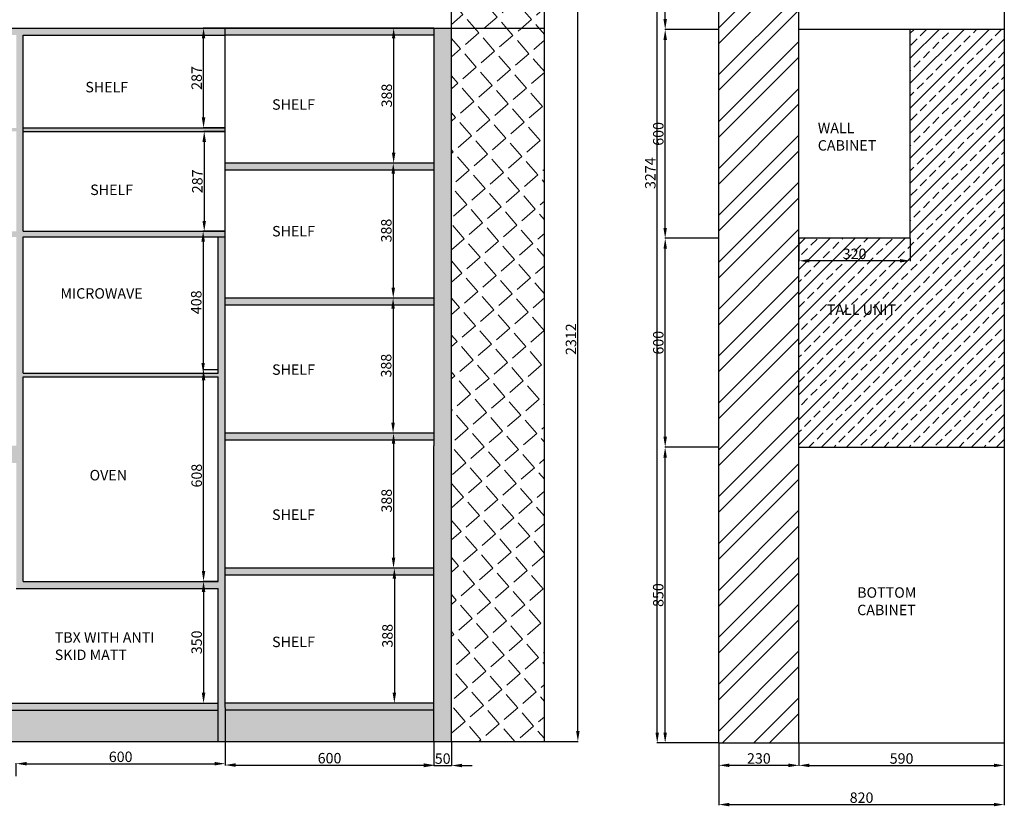
# Model space of a CAD drawing. Units: millimetres. Extents: x 207 to 10383, y -313 to 3598.
# Tile 4 of 5: x 7555 to 10383, y -208 to 2052. Entities that reach past the tile are written whole.
import ezdxf

# ---------------------------------------------------------------- set-up
doc = ezdxf.new("R2010")
doc.units = ezdxf.units.MM
for name, color, linetype, lineweight in [('A-ANNO-DIMS', 2, 'Continuous', 18), ('A-ANNO-TEXT', 3, 'Continuous', 18), ('A-FURN', 7, 'Continuous', 25), ('A-FURN-PATT', 252, 'Continuous', 13), ('A-WALL-PATT', 8, 'Continuous', 13)]:
    doc.layers.add(name, color=color, linetype=linetype, lineweight=lineweight)
doc.styles.get("Standard").update_dxf_attribs({"font": 'arial.ttf'})
doc.dimstyles.new('ISO-25', dxfattribs={"dimtxt": 30, "dimasz": 30, "dimexe": 1.25, "dimexo": 0.625, "dimtad": 1, "dimtxsty": 'Standard', "dimcen": 2.5, "dimadec": 0, "dimazin": 0, "dimtfac": 1, "dimtmove": 0, "dimatfit": 3, "dimfxl": 1, "dimarcsym": 0})

# ---------------------------------------------------------------- blocks, each defined once
blk = doc.blocks.new('*D1')
at = {"layer": 'A-ANNO-DIMS', "color": 0, "lineweight": -2, "transparency": 16777216}
for p, q in [((9562.7, 823.8), (9407.8, 823.8)), ((9409.1, 3.8), (9409.1, 793.8)), ((9562.7, -26.2), (9407.8, -26.2))]:
    blk.add_line(p, q, dxfattribs=at)
at = {"layer": 'A-ANNO-DIMS', "color": 0, "transparency": 16777216}
for points in [[(9404.1, 793.8), (9414.1, 793.8), (9409.1, 823.8)], [(9404.1, 3.8), (9414.1, 3.8), (9409.1, -26.2)]]:
    blk.add_solid(points, dxfattribs=at)
at = {"layer": 'Defpoints', "color": 0, "transparency": 16777216}
for p in [(9409.1, 823.8), (9563.3, 823.8), (9563.3, -26.2)]:
    blk.add_point(p, dxfattribs=at)
at = {"layer": 'A-ANNO-DIMS', "color": 0, "transparency": 16777216, "insert": (9393.1, 398.8), "char_height": 30, "attachment_point": 5, "rotation": 90}
blk.add_mtext('850', dxfattribs=at)
blk = doc.blocks.new('*D2')
at = {"layer": 'A-ANNO-DIMS', "color": 0, "lineweight": -2, "transparency": 16777216}
for p, q in [((9562.7, 1423.8), (9408, 1423.8)), ((9409.3, 853.8), (9409.3, 1393.8)), ((9562.7, 823.8), (9408, 823.8))]:
    blk.add_line(p, q, dxfattribs=at)
at = {"layer": 'A-ANNO-DIMS', "color": 0, "transparency": 16777216}
for points in [[(9404.3, 1393.8), (9414.3, 1393.8), (9409.3, 1423.8)], [(9404.3, 853.8), (9414.3, 853.8), (9409.3, 823.8)]]:
    blk.add_solid(points, dxfattribs=at)
at = {"layer": 'Defpoints', "color": 0, "transparency": 16777216}
for p in [(9409.3, 1423.8), (9563.3, 1423.8), (9563.3, 823.8)]:
    blk.add_point(p, dxfattribs=at)
at = {"layer": 'A-ANNO-DIMS', "color": 0, "transparency": 16777216, "insert": (9393.3, 1123.8), "char_height": 30, "attachment_point": 5, "rotation": 90}
blk.add_mtext('600', dxfattribs=at)
blk = doc.blocks.new('*D3')
at = {"layer": 'A-ANNO-DIMS', "color": 0, "lineweight": -2, "transparency": 16777216}
for p, q in [((9562.7, 2023.8), (9408, 2023.8)), ((9409.2, 1453.8), (9409.2, 1993.8)), ((9562.7, 1423.8), (9408, 1423.8))]:
    blk.add_line(p, q, dxfattribs=at)
at = {"layer": 'A-ANNO-DIMS', "color": 0, "transparency": 16777216}
for points in [[(9404.2, 1993.8), (9414.2, 1993.8), (9409.2, 2023.8)], [(9404.2, 1453.8), (9414.2, 1453.8), (9409.2, 1423.8)]]:
    blk.add_solid(points, dxfattribs=at)
at = {"layer": 'Defpoints', "color": 0, "transparency": 16777216}
for p in [(9409.2, 2023.8), (9563.3, 2023.8), (9563.3, 1423.8)]:
    blk.add_point(p, dxfattribs=at)
at = {"layer": 'A-ANNO-DIMS', "color": 0, "transparency": 16777216, "insert": (9393.3, 1723.8), "char_height": 30, "attachment_point": 5, "rotation": 90}
blk.add_mtext('600', dxfattribs=at)
blk = doc.blocks.new('*D4')
at = {"layer": 'A-ANNO-DIMS', "color": 0, "lineweight": -2, "transparency": 16777216}
for p, q in [((9562.7, 2905.8), (9407.9, 2905.8)), ((9409.2, 2053.8), (9409.2, 2875.8)), ((9562.7, 2023.8), (9407.9, 2023.8))]:
    blk.add_line(p, q, dxfattribs=at)
at = {"layer": 'A-ANNO-DIMS', "color": 0, "transparency": 16777216}
for points in [[(9404.2, 2875.8), (9414.2, 2875.8), (9409.2, 2905.8)], [(9404.2, 2053.8), (9414.2, 2053.8), (9409.2, 2023.8)]]:
    blk.add_solid(points, dxfattribs=at)
at = {"layer": 'Defpoints', "color": 0, "transparency": 16777216}
for p in [(9409.2, 2905.8), (9563.3, 2905.8), (9563.3, 2023.8)]:
    blk.add_point(p, dxfattribs=at)
at = {"layer": 'A-ANNO-DIMS', "color": 0, "transparency": 16777216, "insert": (9393.2, 2464.8), "char_height": 30, "attachment_point": 5, "rotation": 90}
blk.add_mtext('882', dxfattribs=at)
blk = doc.blocks.new('*D7')
at = {"layer": 'A-ANNO-DIMS', "color": 0, "lineweight": -2, "transparency": 16777216}
for p, q in [((9793.3, 1423.2), (9793.3, 1358)), ((10113.3, 1423.2), (10113.3, 1358)), ((10083.3, 1359.2), (9823.3, 1359.2))]:
    blk.add_line(p, q, dxfattribs=at)
at = {"layer": 'A-ANNO-DIMS', "color": 0, "transparency": 16777216}
for points in [[(9823.3, 1364.2), (9823.3, 1354.2), (9793.3, 1359.2)], [(10083.3, 1364.2), (10083.3, 1354.2), (10113.3, 1359.2)]]:
    blk.add_solid(points, dxfattribs=at)
at = {"layer": 'Defpoints', "color": 0, "transparency": 16777216}
for p in [(9793.3, 1423.8), (10113.3, 1423.8), (9793.3, 1359.2)]:
    blk.add_point(p, dxfattribs=at)
at = {"layer": 'A-ANNO-DIMS', "color": 0, "transparency": 16777216, "insert": (9953.3, 1375.2), "char_height": 30, "attachment_point": 5}
blk.add_mtext('320', dxfattribs=at)
blk = doc.blocks.new('*D9')
at = {"layer": 'A-ANNO-DIMS', "color": 0, "lineweight": -2, "transparency": 16777216}
for p, q in [((9563.3, -26.8), (9563.3, -91.7)), ((9793.3, -26.8), (9793.3, -91.7)), ((9593.3, -90.4), (9763.3, -90.4))]:
    blk.add_line(p, q, dxfattribs=at)
at = {"layer": 'A-ANNO-DIMS', "color": 0, "transparency": 16777216}
for points in [[(9593.3, -85.4), (9593.3, -95.4), (9563.3, -90.4)], [(9763.3, -85.4), (9763.3, -95.4), (9793.3, -90.4)]]:
    blk.add_solid(points, dxfattribs=at)
at = {"layer": 'Defpoints', "color": 0, "transparency": 16777216}
for p in [(9563.3, -26.2), (9793.3, -26.2), (9793.3, -90.4)]:
    blk.add_point(p, dxfattribs=at)
at = {"layer": 'A-ANNO-DIMS', "color": 0, "transparency": 16777216, "insert": (9678.3, -74.5), "char_height": 30, "attachment_point": 5}
blk.add_mtext('230', dxfattribs=at)
blk = doc.blocks.new('*D10')
at = {"layer": 'A-ANNO-DIMS', "color": 0, "lineweight": -2, "transparency": 16777216}
for p, q in [((9793.3, -26.8), (9793.3, -91.9)), ((10383.3, -26.8), (10383.3, -91.9)), ((9823.3, -90.6), (10353.3, -90.6))]:
    blk.add_line(p, q, dxfattribs=at)
at = {"layer": 'A-ANNO-DIMS', "color": 0, "transparency": 16777216}
for points in [[(9823.3, -85.6), (9823.3, -95.6), (9793.3, -90.6)], [(10353.3, -85.6), (10353.3, -95.6), (10383.3, -90.6)]]:
    blk.add_solid(points, dxfattribs=at)
at = {"layer": 'Defpoints', "color": 0, "transparency": 16777216}
for p in [(9793.3, -26.2), (10383.3, -26.2), (10383.3, -90.6)]:
    blk.add_point(p, dxfattribs=at)
at = {"layer": 'A-ANNO-DIMS', "color": 0, "transparency": 16777216, "insert": (10088.3, -74.7), "char_height": 30, "attachment_point": 5}
blk.add_mtext('590', dxfattribs=at)
blk = doc.blocks.new('*D47')
at = {"layer": 'A-ANNO-DIMS', "color": 0, "lineweight": -2, "transparency": 16777216}
for p, q in [((8145.1, 75.2), (8145.1, -87)), ((7545.1, -121.5), (7545.1, -84.5)), ((7575.1, -85.7), (8115.1, -85.7))]:
    blk.add_line(p, q, dxfattribs=at)
at = {"layer": 'A-ANNO-DIMS', "color": 0, "transparency": 16777216}
for points in [[(7575.1, -80.7), (7575.1, -90.7), (7545.1, -85.7)], [(8115.1, -80.7), (8115.1, -90.7), (8145.1, -85.7)]]:
    blk.add_solid(points, dxfattribs=at)
at = {"layer": 'Defpoints', "color": 0, "transparency": 16777216}
for p in [(8145.1, 75.9), (8145.1, -85.7), (7545.1, -122.1)]:
    blk.add_point(p, dxfattribs=at)
at = {"layer": 'A-ANNO-DIMS', "color": 0, "transparency": 16777216, "insert": (7845.1, -69.8), "char_height": 30, "attachment_point": 5}
blk.add_mtext('600', dxfattribs=at)
blk = doc.blocks.new('*D48')
at = {"layer": 'A-ANNO-DIMS', "color": 0, "lineweight": -2, "transparency": 16777216}
for p, q in [((8145.1, -22.8), (8145.1, -90.8)), ((8745.1, -22.8), (8745.1, -90.8)), ((8175.1, -89.6), (8715.1, -89.6))]:
    blk.add_line(p, q, dxfattribs=at)
at = {"layer": 'A-ANNO-DIMS', "color": 0, "transparency": 16777216}
for points in [[(8175.1, -84.6), (8175.1, -94.6), (8145.1, -89.6)], [(8715.1, -84.6), (8715.1, -94.6), (8745.1, -89.6)]]:
    blk.add_solid(points, dxfattribs=at)
at = {"layer": 'Defpoints', "color": 0, "transparency": 16777216}
for p in [(8145.1, -22.1), (8745.1, -22.1), (8745.1, -89.6)]:
    blk.add_point(p, dxfattribs=at)
at = {"layer": 'A-ANNO-DIMS', "color": 0, "transparency": 16777216, "insert": (8445.1, -73.7), "char_height": 30, "attachment_point": 5}
blk.add_mtext('600', dxfattribs=at)
blk = doc.blocks.new('*D49')
at = {"layer": 'A-ANNO-DIMS', "color": 0, "lineweight": -2, "transparency": 16777216}
for p, q in [((8745.1, -22.8), (8745.1, -92.2)), ((8795.1, -22.8), (8795.1, -92.2)), ((8715.1, -91), (8685.1, -91)), ((8745.1, -91), (8795.1, -91)), ((8825.1, -91), (8855.1, -91))]:
    blk.add_line(p, q, dxfattribs=at)
at = {"layer": 'A-ANNO-DIMS', "color": 0, "transparency": 16777216}
for points in [[(8715.1, -86), (8715.1, -96), (8745.1, -91)], [(8825.1, -86), (8825.1, -96), (8795.1, -91)]]:
    blk.add_solid(points, dxfattribs=at)
at = {"layer": 'Defpoints', "color": 0, "transparency": 16777216}
for p in [(8745.1, -22.1), (8795.1, -22.1), (8795.1, -91)]:
    blk.add_point(p, dxfattribs=at)
at = {"layer": 'A-ANNO-DIMS', "color": 0, "transparency": 16777216, "insert": (8770.1, -75), "char_height": 30, "attachment_point": 5}
blk.add_mtext('50', dxfattribs=at)
blk = doc.blocks.new('*D58')
at = {"layer": 'A-ANNO-DIMS', "color": 0, "lineweight": -2, "ltscale": 0.3, "transparency": 16777216}
for p, q in [((9063.2, 2289.9), (9159.7, 2289.9)), ((9158.4, 7.9), (9158.4, 2259.9)), ((9063.2, -22.1), (9159.7, -22.1))]:
    blk.add_line(p, q, dxfattribs=at)
at = {"layer": 'A-ANNO-DIMS', "color": 0, "ltscale": 0.3, "transparency": 16777216}
for points in [[(9153.4, 2259.9), (9163.4, 2259.9), (9158.4, 2289.9)], [(9153.4, 7.9), (9163.4, 7.9), (9158.4, -22.1)]]:
    blk.add_solid(points, dxfattribs=at)
at = {"layer": 'Defpoints', "color": 0, "ltscale": 0.3, "transparency": 16777216}
for p in [(9062.5, 2289.9), (9158.4, 2289.9), (9062.5, -22.1)]:
    blk.add_point(p, dxfattribs=at)
at = {"layer": 'A-ANNO-DIMS', "color": 0, "ltscale": 0.3, "transparency": 16777216, "insert": (9142.4, 1133.9), "char_height": 30, "attachment_point": 5, "rotation": 90}
blk.add_mtext('2312', dxfattribs=at)
blk = doc.blocks.new('*D60')
at = {"layer": 'A-ANNO-DIMS', "color": 0, "lineweight": -2, "ltscale": 0.3, "transparency": 16777216}
for p, q in [((8144.4, 2027.9), (8082, 2027.9)), ((8083.2, 1770.9), (8083.2, 1997.9)), ((8144.4, 1740.9), (8082, 1740.9))]:
    blk.add_line(p, q, dxfattribs=at)
at = {"layer": 'A-ANNO-DIMS', "color": 0, "ltscale": 0.3, "transparency": 16777216}
for points in [[(8078.2, 1997.9), (8088.2, 1997.9), (8083.2, 2027.9)], [(8078.2, 1770.9), (8088.2, 1770.9), (8083.2, 1740.9)]]:
    blk.add_solid(points, dxfattribs=at)
at = {"layer": 'Defpoints', "color": 0, "ltscale": 0.3, "transparency": 16777216}
for p in [(8083.2, 2027.9), (8145.1, 2027.9), (8145.1, 1740.9)]:
    blk.add_point(p, dxfattribs=at)
at = {"layer": 'A-ANNO-DIMS', "color": 0, "ltscale": 0.3, "transparency": 16777216, "insert": (8067.3, 1884.4), "char_height": 30, "attachment_point": 5, "rotation": 90}
blk.add_mtext('287', dxfattribs=at)
blk = doc.blocks.new('*D59')
at = {"layer": 'A-ANNO-DIMS', "color": 0, "lineweight": -2, "ltscale": 0.3, "transparency": 16777216}
for p, q in [((8124.4, 1045.9), (8082, 1045.9)), ((8083.2, 467.9), (8083.2, 1015.9)), ((8124.4, 437.9), (8082, 437.9))]:
    blk.add_line(p, q, dxfattribs=at)
at = {"layer": 'A-ANNO-DIMS', "color": 0, "ltscale": 0.3, "transparency": 16777216}
for points in [[(8078.2, 1015.9), (8088.2, 1015.9), (8083.2, 1045.9)], [(8078.2, 467.9), (8088.2, 467.9), (8083.2, 437.9)]]:
    blk.add_solid(points, dxfattribs=at)
at = {"layer": 'Defpoints', "color": 0, "ltscale": 0.3, "transparency": 16777216}
for p in [(8083.2, 1045.9), (8125.1, 1045.9), (8125.1, 437.9)]:
    blk.add_point(p, dxfattribs=at)
at = {"layer": 'A-ANNO-DIMS', "color": 0, "ltscale": 0.3, "transparency": 16777216, "insert": (8067.3, 741.9), "char_height": 30, "attachment_point": 5, "rotation": 90}
blk.add_mtext('608', dxfattribs=at)
blk = doc.blocks.new('*D61')
at = {"layer": 'A-ANNO-DIMS', "color": 0, "lineweight": -2, "ltscale": 0.3, "transparency": 16777216}
for p, q in [((8144.4, 1730.9), (8083.9, 1730.9)), ((8085.1, 1700.9), (8085.1, 1473.9)), ((8144.4, 1443.9), (8083.9, 1443.9))]:
    blk.add_line(p, q, dxfattribs=at)
at = {"layer": 'A-ANNO-DIMS', "color": 0, "ltscale": 0.3, "transparency": 16777216}
for points in [[(8080.1, 1700.9), (8090.1, 1700.9), (8085.1, 1730.9)], [(8080.1, 1473.9), (8090.1, 1473.9), (8085.1, 1443.9)]]:
    blk.add_solid(points, dxfattribs=at)
at = {"layer": 'Defpoints', "color": 0, "ltscale": 0.3, "transparency": 16777216}
for p in [(8145.1, 1730.9), (8085.1, 1443.9), (8145.1, 1443.9)]:
    blk.add_point(p, dxfattribs=at)
at = {"layer": 'A-ANNO-DIMS', "color": 0, "ltscale": 0.3, "transparency": 16777216, "insert": (8069.2, 1587.4), "char_height": 30, "attachment_point": 5, "rotation": 90}
blk.add_mtext('287', dxfattribs=at)
blk = doc.blocks.new('*D62')
at = {"layer": 'A-ANNO-DIMS', "color": 0, "lineweight": -2, "ltscale": 0.3, "transparency": 16777216}
for p, q in [((8084.5, 1443.9), (8080.7, 1443.9)), ((8082, 1413.9), (8082, 1065.9)), ((8084.3, 1035.9), (8080.7, 1035.9))]:
    blk.add_line(p, q, dxfattribs=at)
at = {"layer": 'A-ANNO-DIMS', "color": 0, "ltscale": 0.3, "transparency": 16777216}
for points in [[(8077, 1413.9), (8087, 1413.9), (8082, 1443.9)], [(8077, 1065.9), (8087, 1065.9), (8082, 1035.9)]]:
    blk.add_solid(points, dxfattribs=at)
at = {"layer": 'Defpoints', "color": 0, "ltscale": 0.3, "transparency": 16777216}
for p in [(8085.1, 1443.9), (8082, 1035.9), (8084.9, 1035.9)]:
    blk.add_point(p, dxfattribs=at)
at = {"layer": 'A-ANNO-DIMS', "color": 0, "ltscale": 0.3, "transparency": 16777216, "insert": (8066.1, 1239.9), "char_height": 30, "attachment_point": 5, "rotation": 90}
blk.add_mtext('408', dxfattribs=at)
blk = doc.blocks.new('*D63')
at = {"layer": 'A-ANNO-DIMS', "color": 0, "lineweight": -2, "ltscale": 0.3, "transparency": 16777216}
for p, q in [((8083.9, 437.9), (8084.5, 437.9)), ((8083.2, 407.9), (8083.2, 117.9)), ((8083.9, 87.9), (8084.5, 87.9))]:
    blk.add_line(p, q, dxfattribs=at)
at = {"layer": 'A-ANNO-DIMS', "color": 0, "ltscale": 0.3, "transparency": 16777216}
for points in [[(8078.2, 407.9), (8088.2, 407.9), (8083.2, 437.9)], [(8078.2, 117.9), (8088.2, 117.9), (8083.2, 87.9)]]:
    blk.add_solid(points, dxfattribs=at)
at = {"layer": 'Defpoints', "color": 0, "ltscale": 0.3, "transparency": 16777216}
for p in [(8083.2, 437.9), (8083.2, 87.9), (8083.2, 87.9)]:
    blk.add_point(p, dxfattribs=at)
at = {"layer": 'A-ANNO-DIMS', "color": 0, "ltscale": 0.3, "transparency": 16777216, "insert": (8067.3, 262.9), "char_height": 30, "attachment_point": 5, "rotation": 90}
blk.add_mtext('350', dxfattribs=at)
blk = doc.blocks.new('*D64')
at = {"layer": 'A-ANNO-DIMS', "color": 0, "lineweight": -2, "ltscale": 0.3, "transparency": 16777216}
for p, q in [((8744.4, 2027.9), (8628, 2027.9)), ((8629.2, 1997.9), (8629.2, 1669.9)), ((8744.4, 1639.9), (8628, 1639.9))]:
    blk.add_line(p, q, dxfattribs=at)
at = {"layer": 'A-ANNO-DIMS', "color": 0, "ltscale": 0.3, "transparency": 16777216}
for points in [[(8624.2, 1997.9), (8634.2, 1997.9), (8629.2, 2027.9)], [(8624.2, 1669.9), (8634.2, 1669.9), (8629.2, 1639.9)]]:
    blk.add_solid(points, dxfattribs=at)
at = {"layer": 'Defpoints', "color": 0, "ltscale": 0.3, "transparency": 16777216}
for p in [(8745.1, 2027.9), (8629.2, 1639.9), (8745.1, 1639.9)]:
    blk.add_point(p, dxfattribs=at)
at = {"layer": 'A-ANNO-DIMS', "color": 0, "ltscale": 0.3, "transparency": 16777216, "insert": (8613.3, 1833.9), "char_height": 30, "attachment_point": 5, "rotation": 90}
blk.add_mtext('388', dxfattribs=at)
blk = doc.blocks.new('*D65')
at = {"layer": 'A-ANNO-DIMS', "color": 0, "lineweight": -2, "ltscale": 0.3, "transparency": 16777216}
for p, q in [((8744.4, 1639.9), (8626.8, 1639.9)), ((8628.1, 1609.9), (8628.1, 1281.9)), ((8744.4, 1251.9), (8626.8, 1251.9))]:
    blk.add_line(p, q, dxfattribs=at)
at = {"layer": 'A-ANNO-DIMS', "color": 0, "ltscale": 0.3, "transparency": 16777216}
for points in [[(8623.1, 1609.9), (8633.1, 1609.9), (8628.1, 1639.9)], [(8623.1, 1281.9), (8633.1, 1281.9), (8628.1, 1251.9)]]:
    blk.add_solid(points, dxfattribs=at)
at = {"layer": 'Defpoints', "color": 0, "ltscale": 0.3, "transparency": 16777216}
for p in [(8745.1, 1639.9), (8628.1, 1251.9), (8745.1, 1251.9)]:
    blk.add_point(p, dxfattribs=at)
at = {"layer": 'A-ANNO-DIMS', "color": 0, "ltscale": 0.3, "transparency": 16777216, "insert": (8612.1, 1445.9), "char_height": 30, "attachment_point": 5, "rotation": 90}
blk.add_mtext('388', dxfattribs=at)
blk = doc.blocks.new('*D66')
at = {"layer": 'A-ANNO-DIMS', "color": 0, "lineweight": -2, "ltscale": 0.3, "transparency": 16777216}
for p, q in [((8744.4, 1251.9), (8626.4, 1251.9)), ((8627.6, 1221.9), (8627.6, 893.9)), ((8744.4, 863.9), (8626.4, 863.9))]:
    blk.add_line(p, q, dxfattribs=at)
at = {"layer": 'A-ANNO-DIMS', "color": 0, "ltscale": 0.3, "transparency": 16777216}
for points in [[(8622.6, 1221.9), (8632.6, 1221.9), (8627.6, 1251.9)], [(8622.6, 893.9), (8632.6, 893.9), (8627.6, 863.9)]]:
    blk.add_solid(points, dxfattribs=at)
at = {"layer": 'Defpoints', "color": 0, "ltscale": 0.3, "transparency": 16777216}
for p in [(8745.1, 1251.9), (8627.6, 863.9), (8745.1, 863.9)]:
    blk.add_point(p, dxfattribs=at)
at = {"layer": 'A-ANNO-DIMS', "color": 0, "ltscale": 0.3, "transparency": 16777216, "insert": (8611.7, 1057.9), "char_height": 30, "attachment_point": 5, "rotation": 90}
blk.add_mtext('388', dxfattribs=at)
blk = doc.blocks.new('*D67')
at = {"layer": 'A-ANNO-DIMS', "color": 0, "lineweight": -2, "ltscale": 0.3, "transparency": 16777216}
for p, q in [((8744.4, 863.9), (8627.6, 863.9)), ((8628.9, 833.9), (8628.9, 505.9)), ((8744.4, 475.9), (8627.6, 475.9))]:
    blk.add_line(p, q, dxfattribs=at)
at = {"layer": 'A-ANNO-DIMS', "color": 0, "ltscale": 0.3, "transparency": 16777216}
for points in [[(8623.9, 833.9), (8633.9, 833.9), (8628.9, 863.9)], [(8623.9, 505.9), (8633.9, 505.9), (8628.9, 475.9)]]:
    blk.add_solid(points, dxfattribs=at)
at = {"layer": 'Defpoints', "color": 0, "ltscale": 0.3, "transparency": 16777216}
for p in [(8745.1, 863.9), (8628.9, 475.9), (8745.1, 475.9)]:
    blk.add_point(p, dxfattribs=at)
at = {"layer": 'A-ANNO-DIMS', "color": 0, "ltscale": 0.3, "transparency": 16777216, "insert": (8612.9, 669.9), "char_height": 30, "attachment_point": 5, "rotation": 90}
blk.add_mtext('388', dxfattribs=at)
blk = doc.blocks.new('*D68')
at = {"layer": 'A-ANNO-DIMS', "color": 0, "lineweight": -2, "ltscale": 0.3, "transparency": 16777216}
for p, q in [((8744.4, 475.9), (8630, 475.9)), ((8631.3, 445.9), (8631.3, 117.9)), ((8744.4, 87.9), (8630, 87.9))]:
    blk.add_line(p, q, dxfattribs=at)
at = {"layer": 'A-ANNO-DIMS', "color": 0, "ltscale": 0.3, "transparency": 16777216}
for points in [[(8626.3, 445.9), (8636.3, 445.9), (8631.3, 475.9)], [(8626.3, 117.9), (8636.3, 117.9), (8631.3, 87.9)]]:
    blk.add_solid(points, dxfattribs=at)
at = {"layer": 'Defpoints', "color": 0, "ltscale": 0.3, "transparency": 16777216}
for p in [(8745.1, 475.9), (8631.3, 87.9), (8745.1, 87.9)]:
    blk.add_point(p, dxfattribs=at)
at = {"layer": 'A-ANNO-DIMS', "color": 0, "ltscale": 0.3, "transparency": 16777216, "insert": (8615.3, 281.9), "char_height": 30, "attachment_point": 5, "rotation": 90}
blk.add_mtext('388', dxfattribs=at)
blk = doc.blocks.new('*D95')
at = {"layer": 'A-ANNO-DIMS', "color": 0, "lineweight": -2, "ltscale": 0.3, "transparency": 16777216}
for p, q in [((9562.7, 3247.8), (9385.1, 3247.8)), ((9386.3, 3.8), (9386.3, 3217.8)), ((9562.7, -26.2), (9385.1, -26.2))]:
    blk.add_line(p, q, dxfattribs=at)
at = {"layer": 'A-ANNO-DIMS', "color": 0, "ltscale": 0.3, "transparency": 16777216}
for points in [[(9381.3, 3217.8), (9391.3, 3217.8), (9386.3, 3247.8)], [(9381.3, 3.8), (9391.3, 3.8), (9386.3, -26.2)]]:
    blk.add_solid(points, dxfattribs=at)
at = {"layer": 'Defpoints', "color": 0, "ltscale": 0.3, "transparency": 16777216}
for p in [(9386.3, 3247.8), (9563.3, 3247.8), (9563.3, -26.2)]:
    blk.add_point(p, dxfattribs=at)
at = {"layer": 'A-ANNO-DIMS', "color": 0, "ltscale": 0.3, "transparency": 16777216, "insert": (9370.4, 1610.8), "char_height": 30, "attachment_point": 5, "rotation": 90}
blk.add_mtext('3274', dxfattribs=at)
blk = doc.blocks.new('*D96')
at = {"layer": 'A-ANNO-DIMS', "color": 0, "lineweight": -2, "ltscale": 0.3, "transparency": 16777216}
for p, q in [((9563.3, -26.8), (9563.3, -204.4)), ((10383.3, -26.8), (10383.3, -204.4)), ((9593.3, -203.2), (10353.3, -203.2))]:
    blk.add_line(p, q, dxfattribs=at)
at = {"layer": 'A-ANNO-DIMS', "color": 0, "ltscale": 0.3, "transparency": 16777216}
for points in [[(9593.3, -198.2), (9593.3, -208.2), (9563.3, -203.2)], [(10353.3, -198.2), (10353.3, -208.2), (10383.3, -203.2)]]:
    blk.add_solid(points, dxfattribs=at)
at = {"layer": 'Defpoints', "color": 0, "ltscale": 0.3, "transparency": 16777216}
for p in [(9563.3, -26.2), (10383.3, -26.2), (10383.3, -203.2)]:
    blk.add_point(p, dxfattribs=at)
at = {"layer": 'A-ANNO-DIMS', "color": 0, "ltscale": 0.3, "transparency": 16777216, "insert": (9973.3, -187.2), "char_height": 30, "attachment_point": 5}
blk.add_mtext('820', dxfattribs=at)

msp = doc.modelspace()

# ---------------------------------------------------------------- hatches: boundary and pattern name
at = {"layer": 'A-FURN-PATT', "ltscale": 0.3}
h = msp.add_hatch(color=256, dxfattribs=at)
h.dxf.hatch_style = 1
h.paths.add_polyline_path([(7545.0576, 827.8543), (6103.7405, 827.8543), (6103.7405, 777.8543), (7545.0576, 777.8543)])
h.paths.add_polyline_path([(6103.7405, 827.8543), (5302.0576, 827.8543), (5302.0576, 777.8543), (6103.7405, 777.8543)])
h.paths.add_polyline_path([(6355.0576, 777.8543), (6335.0576, 777.8543), (6335.0576, 87.8543), (5302.0576, 87.8543), (5302.0576, 67.8543), (7265.0576, 67.8543), (7265.0576, 777.8543), (7245.0576, 777.8543), (7245.0576, 87.8543), (6355.0576, 87.8543)])
h.paths.add_polyline_path([(8145.0576, 1427.8543), (8125.0576, 1427.8543), (8125.0576, 1035.8543), (7565.0576, 1035.8543), (7565.0576, 1427.8543), (8145.0576, 1427.8543), (8145.0576, 1443.8543), (7565.0576, 1443.8543), (7565.0576, 2007.8543), (8145.0576, 2007.8543), (8145.0576, 2027.8543), (7374.0165, 2027.8543), (7374.0165, 2007.8543), (7545.0576, 2007.8543), (7545.0576, 1443.8543), (7265.0576, 1443.8543), (7265.0576, 1427.8543), (7545.0576, 1427.8543), (7545.0576, 417.8543), (8125.0576, 417.8543), (8125.0576, -22.1457), (8745.0576, -22.1457), (8745.0576, 87.8543), (8145.0576, 87.8543)])
h.paths.add_polyline_path([(7565.0576, 437.8543), (7565.0576, 1025.8543), (8125.0576, 1025.8543), (8125.0576, 437.8543)], flags=16)
h.paths.add_polyline_path([(8125.0576, 67.8543), (5302.0576, 67.8543), (5302.0576, -22.1457), (5892.0576, -22.1457), (8125.0576, -22.1457)])
h.paths.add_polyline_path([(8125.0576, 87.8543), (7265.0576, 87.8543), (7265.0576, 67.8543), (8125.0576, 67.8543)], flags=17)
h.paths.add_polyline_path([(8745.0576, 475.8543), (8145.0576, 475.8543), (8145.0576, 455.8543), (8745.0576, 455.8543)], flags=17)
h.paths.add_polyline_path([(8745.0576, 863.8543), (8145.0576, 863.8543), (8145.0576, 843.8543), (8745.0576, 843.8543)], flags=17)
h.paths.add_polyline_path([(8745.0576, 1251.8543), (8145.0576, 1251.8543), (8145.0576, 1231.8543), (8745.0576, 1231.8543)])
h.paths.add_polyline_path([(8745.0576, 1639.8543), (8145.0576, 1639.8543), (8145.0576, 1619.8543), (8745.0576, 1619.8543)])
h.paths.add_polyline_path([(7545.0576, 1740.8543), (7265.0576, 1740.8543), (7265.0576, 1730.8543), (7545.0576, 1730.8543)], flags=17)
h.paths.add_polyline_path([(8145.0576, 1740.8543), (7565.0576, 1740.8543), (7565.0576, 1730.8543), (8145.0576, 1730.8543)], flags=17)
h.paths.add_polyline_path([(7265.0576, 2007.8543), (7374.0165, 2007.8543), (7374.0165, 2027.8543), (7245.0576, 2027.8543), (7245.0576, 1427.8543), (7265.0576, 1427.8543), (7265.0576, 1443.8543)])
h.paths.add_polyline_path([(8745.0576, 2027.8543), (8145.0576, 2027.8543), (8145.0576, 2007.8543), (8745.0576, 2007.8543)])
h.paths.add_polyline_path([(8795.0576, 2027.8543), (8745.0576, 2027.8543), (8745.0576, 2007.8543), (8745.0576, 827.8543), (8745.0576, -22.1457), (8795.0576, -22.1457)])
h.paths.add_polyline_path([(6275.0576, 2027.8543), (5302.0576, 2027.8543), (5302.0576, 1427.8543), (6275.0576, 1427.8543), (6275.0576, 2007.8543), (6255.0576, 2007.8543), (6255.0576, 1443.8543), (5955.0576, 1443.8543), (5955.0576, 2007.8543), (5935.0576, 2007.8543), (5935.0576, 1443.8543), (5312.0576, 1443.8543), (5312.0576, 2007.8543), (6275.0576, 2007.8543)])
h.paths.add_polyline_path([(5935.0576, 1740.8543), (5312.0576, 1740.8543), (5312.0576, 1730.8543), (5935.0576, 1730.8543)], flags=17)
h.paths.add_polyline_path([(6255.0576, 1740.8543), (5955.0576, 1740.8543), (5955.0576, 1730.8543), (6255.0576, 1730.8543)], flags=17)
h.paths.add_polyline_path([(7746.303, 711.3558), (7880.0751, 711.3558), (7880.0751, 773.177), (7746.303, 773.177)], flags=8)
h.paths.add_polyline_path([(6298.0591, -5.5925), (6676.3333, -5.5925), (6676.3333, 56.2287), (6298.0591, 56.2287)], flags=24)
at = {"layer": 'A-FURN-PATT'}
h = msp.add_hatch(dxfattribs=at)
h.set_pattern_fill('ANSI33', color=256, scale=8)
h.set_pattern_definition([(45, (1161.48, -1119.74), (-35.92102, 35.92102), []), (45, (1197.4, -1119.74), (-35.92102, 35.92102), [25.4, -12.7])])
h.paths.add_polyline_path([(9793.3374, 823.8417), (10383.3374, 823.8417), (10383.3374, 2023.8417), (10113.3374, 2023.8417), (10113.3374, 1423.8417), (9793.3374, 1423.8417)])
h.paths.add_polyline_path([(9910.9977, 1344.0012), (9995.9227, 1344.0012), (9995.9227, 1405.8225), (9910.9977, 1405.8225)], flags=24)
h.paths.add_polyline_path([(9865.1294, 1187.4265), (10089.7201, 1187.4265), (10089.7201, 1249.2477), (9865.1294, 1249.2477)], flags=24)
at = {"layer": 'A-WALL-PATT'}
h = msp.add_hatch(dxfattribs=at)
h.set_pattern_fill('ANSI32', color=256, scale=10)
h.set_pattern_definition([(45, (1161.48, -1119.74), (-67.3519, 67.3519), []), (45, (1206.38, -1119.74), (-67.3519, 67.3519), [])])
h.paths.add_polyline_path([(9793.3374, 2905.8417), (9793.3374, 3247.8417), (9563.3374, 3247.8417), (9563.3374, 2905.8417), (9563.3374, -26.1583), (9793.3374, -26.1583)])
h = msp.add_hatch(dxfattribs=at)
h.set_pattern_fill('ANGLE', color=256, scale=10, angle=131)
h.set_pattern_definition([(131, (2244.98, -3563.3), (-52.71646, -45.8257), [50.8, -19.05]), (221, (2244.98, -3563.3), (45.8257, -52.71646), [50.8, -19.05])])
h.paths.add_polyline_path([(9062.5445, 2289.8543), (8795.0576, 2289.8543), (8795.0576, -22.1457), (9062.5445, -22.1457)])

# ---------------------------------------------------------------- linework, layer by layer
at = {"layer": 'A-FURN'}
for p, q in [((8795.0576, -22.1457), (8795.0576, 2911.8543)), ((9062.5445, -22.1457), (9062.5445, 2911.8543)), ((9563.3374, -26.1583), (9563.3374, 2905.8417)), ((9793.3374, -26.1583), (9793.3374, 2905.8417)), ((10383.3374, 2905.8417), (10383.3374, -26.1583)), ((5302.0576, 2027.8543), (9062.5445, 2027.8543)), ((8145.0576, 75.8543), (8145.0576, 2027.8543)), ((8745.0576, 2027.8543), (8745.0576, 827.8543)), ((10383.3374, 2023.8417), (9793.3374, 2023.8417)), ((10113.3374, 1423.8417), (10113.3374, 2023.8417)), ((7565.0576, 1443.8543), (7565.0576, 2007.8543)), ((7565.0576, 1740.8543), (8145.0576, 1740.8543)), ((7565.0576, 1730.8543), (8145.0576, 1730.8543)), ((7565.0576, 1443.8543), (8145.0576, 1443.8543)), ((7565.0576, 1035.8543), (7565.0576, 1427.8543)), ((7565.0576, 1427.8543), (8145.0576, 1427.8543)), ((8125.0576, 1035.8543), (8125.0576, 1427.8543)), ((10113.3374, 1423.8417), (9793.3374, 1423.8417)), ((7565.0576, 1035.8543), (8125.0576, 1035.8543)), ((7565.0576, 437.8543), (7565.0576, 1025.8543)), ((8125.0576, 437.8543), (8125.0576, 1025.8543)), ((8745.0576, -22.1457), (8745.0576, 827.8543)), ((9793.3374, 823.8417), (10383.3374, 823.8417)), ((8125.0576, -22.1457), (8125.0576, 417.8543)), ((5892.0576, -22.1457), (9062.5445, -22.1457)), ((9563.3374, -26.1583), (10383.3374, -26.1583))]:
    msp.add_line(p, q, dxfattribs=at)
at = {"layer": 'A-FURN', "ltscale": 0.3}
for p, q in [((8745.0576, 2027.8543), (8145.0576, 2027.8543)), ((7565.0576, 2007.8543), (8145.0576, 2007.8543)), ((8745.0576, 2007.8543), (8145.0576, 2007.8543)), ((8745.0576, 1639.8543), (8145.0576, 1639.8543)), ((8745.0576, 1619.8543), (8145.0576, 1619.8543)), ((7565.0841, 1423.8544), (7565.0576, 1423.8543)), ((8745.0576, 1251.8543), (8145.0576, 1251.8543)), ((8745.0576, 1231.8543), (8145.0576, 1231.8543)), ((7565.0576, 1025.8543), (8125.0576, 1025.8543)), ((8745.0576, 863.8543), (8145.0576, 863.8543)), ((8745.0576, 843.8543), (8145.0576, 843.8543)), ((8745.0576, 475.8543), (8145.0576, 475.8543)), ((8745.0576, 455.8543), (8145.0576, 455.8543)), ((7565.0576, 437.8543), (8125.0576, 437.8543)), ((7545.0576, 417.8543), (8125.0576, 417.8543)), ((7265.0576, 87.8543), (8125.0576, 87.8543)), ((8745.0576, 87.8543), (8145.0576, 87.8543)), ((5302.0576, 67.8543), (8125.0576, 67.8543)), ((8745.0576, 67.8543), (8145.0576, 67.8543))]:
    msp.add_line(p, q, dxfattribs=at)

# ---------------------------------------------------------------- texts
at = {"layer": 'A-ANNO-TEXT', "ltscale": 0.3, "char_height": 30, "attachment_point": 1}
for s, insert in [('SHELF', (7743.6758, 1873.1105)), ('SHELF', (8280.0135, 1823.1444)), ('SHELF', (7757.6392, 1578.0647)), ('SHELF', (8280.0135, 1459.1693)), ('MICROWAVE', (7672.1382, 1280.4316)), ('SHELF', (8280.0135, 1061.5099)), ('OVEN', (7755.8289, 758.2691)), ('SHELF', (8280.0135, 644.7083)), ('TBX WITH ANTI SKID MATT', (7655.7367, 292.0485)), ('SHELF', (8280.0135, 279.2548))]:
    msp.add_mtext_dynamic_manual_height_columns(s, width=313.278638, gutter_width=12.5, heights=[0], dxfattribs=dict(at, insert=insert))
at = {"layer": 'A-ANNO-TEXT', "char_height": 30, "attachment_point": 1}
for s, insert in [('WALL CABINET', (9847.5514, 1755.7579)), ('TALL UNIT', (9873.6116, 1233.8078)), ('BOTTOM \\PCABINET', (9960.7754, 420.9886))]:
    msp.add_mtext_dynamic_manual_height_columns(s, width=229.851482, gutter_width=12.5, heights=[0], dxfattribs=dict(at, insert=insert))

# ---------------------------------------------------------------- dimensions: what is measured, and where the dimension line sits
at = {"layer": 'A-ANNO-DIMS', "ltscale": 0.3}
for base, p1, p2, override, picture, middle in [((9386.3374, 3247.8417), (9563.3374, -26.1583), (9563.3374, 3247.8417), {"dimdec": 0, "dimlfac": 1, "dimrnd": 0, "dimzin": 0, "dimdsep": 46, "dimlunit": 2}, '*D95', (9370.385, 1610.8417)), ((9158.4022, 2289.8543), (9062.5445, -22.1457), (9062.5445, 2289.8543), {"dimclrd": 0, "dimclre": 0, "dimclrt": 0}, '*D58', (9142.4498, 1133.8543)), ((8083.2454, 2027.8543), (8145.0576, 1740.8543), (8145.0576, 2027.8543), {"dimclrd": 0, "dimclre": 0, "dimclrt": 0}, '*D60', (8067.3032, 1884.3543)), ((8629.2261, 1639.8543), (8745.0576, 2027.8543), (8745.0576, 1639.8543), {"dimclrd": 0, "dimclre": 0, "dimclrt": 0}, '*D64', (8613.2737, 1833.8543)), ((8085.1115, 1443.8543), (8145.0576, 1730.8543), (8145.0576, 1443.8543), {"dimclrd": 0, "dimclre": 0, "dimclrt": 0}, '*D61', (8069.1693, 1587.3543)), ((8628.0548, 1251.8543), (8745.0576, 1639.8543), (8745.0576, 1251.8543), {"dimclrd": 0, "dimclre": 0, "dimclrt": 0}, '*D65', (8612.1024, 1445.8543)), ((8081.9954, 1035.8543), (8085.1115, 1443.8543), (8084.9121, 1035.8543), {"dimclrd": 0, "dimclre": 0, "dimclrt": 0}, '*D62', (8066.0532, 1239.8543)), ((8627.6451, 863.8543), (8745.0576, 1251.8543), (8745.0576, 863.8543), {"dimclrd": 0, "dimclre": 0, "dimclrt": 0}, '*D66', (8611.6927, 1057.8543)), ((8083.2454, 1045.8543), (8125.0576, 437.8543), (8125.0576, 1045.8543), {"dimclrd": 0, "dimclre": 0, "dimclrt": 0}, '*D59', (8067.3032, 741.8543)), ((8628.8732, 475.8543), (8745.0576, 863.8543), (8745.0576, 475.8543), {"dimclrd": 0, "dimclre": 0, "dimclrt": 0}, '*D67', (8612.9207, 669.8543)), ((8631.2659, 87.8543), (8745.0576, 475.8543), (8745.0576, 87.8543), {"dimclrd": 0, "dimclre": 0, "dimclrt": 0}, '*D68', (8615.3135, 281.8543))]:
    dim = msp.add_linear_dim(base=base, p1=p1, p2=p2, angle=90, dimstyle='ISO-25', override=override, dxfattribs=at)
    dim.commit()
    dim.dimension.update_dxf_attribs({"geometry": picture, "text_midpoint": middle})
at = {"layer": 'A-ANNO-DIMS'}
for base, p1, p2, picture, middle in [((9409.1837, 2905.8417), (9563.3374, 2023.8417), (9563.3374, 2905.8417), '*D4', (9393.2415, 2464.8417)), ((9409.2175, 2023.8417), (9563.3374, 1423.8417), (9563.3374, 2023.8417), '*D3', (9393.2753, 1723.8417)), ((9409.2735, 1423.8417), (9563.3374, 823.8417), (9563.3374, 1423.8417), '*D2', (9393.3314, 1123.8417)), ((9409.0697, 823.8417), (9563.3374, -26.1583), (9563.3374, 823.8417), '*D1', (9393.1275, 398.8417))]:
    dim = msp.add_linear_dim(base=base, p1=p1, p2=p2, angle=90, dimstyle='ISO-25', override={"dimclrd": 0, "dimclre": 0, "dimclrt": 0}, dxfattribs=at)
    dim.commit()
    dim.dimension.update_dxf_attribs({"geometry": picture, "text_midpoint": middle})
for base, p1, p2, picture, middle in [((9793.3374, 1359.2255), (10113.3374, 1423.8417), (9793.3374, 1423.8417), '*D7', (9953.3374, 1375.1779)), ((8145.0576, -85.7347), (7545.0576, -122.1457), (8145.0576, 75.8543), '*D47', (7845.0576, -69.7925)), ((8745.0576, -89.5976), (8145.0576, -22.1457), (8745.0576, -22.1457), '*D48', (8445.0576, -73.6554)), ((8795.0576, -90.9872), (8745.0576, -22.1457), (8795.0576, -22.1457), '*D49', (8770.0576, -75.045)), ((9793.3374, -90.4047), (9563.3374, -26.1583), (9793.3374, -26.1583), '*D9', (9678.3374, -74.4522)), ((10383.3374, -90.6308), (9793.3374, -26.1583), (10383.3374, -26.1583), '*D10', (10088.3374, -74.6886))]:
    dim = msp.add_linear_dim(base=base, p1=p1, p2=p2, dimstyle='ISO-25', override={"dimclrd": 0, "dimclre": 0, "dimclrt": 0}, dxfattribs=at)
    dim.commit()
    dim.dimension.update_dxf_attribs({"geometry": picture, "text_midpoint": middle})
at = {"layer": 'A-ANNO-DIMS', "ltscale": 0.3}
dim = msp.add_aligned_dim(p1=(8083.2454, 437.8543), p2=(8083.2454, 87.8543), distance=0, dimstyle='ISO-25', override={"dimclrd": 0, "dimclre": 0, "dimclrt": 0}, dxfattribs=at)
dim.commit()
dim.dimension.update_dxf_attribs({"geometry": '*D63', "text_midpoint": (8067.293, 262.8543)})
dim = msp.add_linear_dim(base=(10383.3374, -203.1583), p1=(9563.3374, -26.1583), p2=(10383.3374, -26.1583), dimstyle='ISO-25', override={"dimdec": 0, "dimlfac": 1, "dimrnd": 0, "dimzin": 0, "dimdsep": 46, "dimlunit": 2}, dxfattribs=at)
dim.commit()
dim.dimension.update_dxf_attribs({"geometry": '*D96', "text_midpoint": (9973.3374, -187.2161)})

doc.saveas('drawing.dxf')
